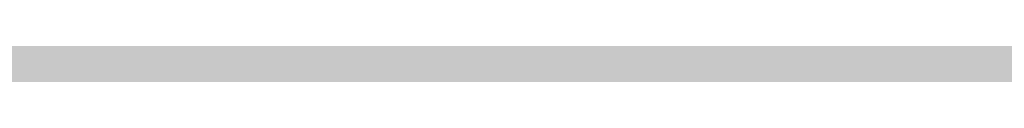
# Model space of a CAD drawing. Units: inches. Extents: x 2091 to 2899, y 967 to 2217.
# Tile 228 of 256: x 2203.4104 to 2203.7172, y 1152.2538 to 1152.2605. Entities that reach past the tile are written whole.
import ezdxf

# ---------------------------------------------------------------- set-up
doc = ezdxf.new("R2010")
doc.units = ezdxf.units.IN
doc.layers.add('A-WALL-PATT', color=141, linetype='Continuous', lineweight=13, true_color=0xadddf7)

msp = doc.modelspace()

# ---------------------------------------------------------------- hatches: boundary and pattern name
at = {"layer": 'A-WALL-PATT'}
h = msp.add_hatch(color=256, dxfattribs=at)
h.dxf.hatch_style = 1
h.paths.add_polyline_path([(2803.1436, 2050.91906), (2203.1436, 2050.91906), (2203.1436, 1090.91906), (2803.1436, 1090.91906)])
h.paths.add_polyline_path([(2635.79885, 1147.54046), (2674.52405, 1147.54046, 0.376086), (2678.52967, 1152.8802), (2678.52967, 1159.55647, 0.333335), (2674.52432, 1163.56185), (2674.52432, 1163.56185), (2674.52432, 1192.93439), (2635.80597, 1192.93439), (2597.08762, 1192.93439), (2597.08762, 1163.56185, 0.333335), (2593.08228, 1159.55647), (2593.08228, 1152.8802, 0.376086), (2597.08789, 1147.54046)], flags=0)
h.paths.add_polyline_path([(2436.01043, 1278.24078, 0.000483), (2435.95264, 1278.21503, -0.001328), (2435.93563, 1278.11169, -0.001711), (2436.11644, 1278.04076, 0.002185)], flags=0)
h.paths.add_polyline_path([(2794.1436, 1143.41906), (2794.1436, 1347.41906), (2543.37017, 1347.41906), (2543.37017, 1351.91906), (2794.1436, 1351.91906), (2794.1436, 1392.71355), (2793.9474, 1392.71355), (2793.9474, 1473.5369), (2794.1436, 1473.5369), (2794.1436, 1531.91906), (2650.1436, 1531.91906), (2650.1436, 1536.41906), (2794.1436, 1536.41906), (2794.1436, 1692.41906), (2609.37561, 1692.41906), (2609.37561, 1644.41906), (2604.87561, 1644.41906), (2604.87561, 1744.91906), (2609.37561, 1744.91906), (2609.37561, 1696.91906), (2794.1436, 1696.91906), (2794.1436, 1780.91906), (2609.6436, 1780.91906), (2493.87561, 1780.91906), (2493.87561, 1785.41906), (2609.6436, 1785.41906), (2794.1436, 1785.41906), (2794.1436, 1847.93882), (2793.95122, 1847.93882), (2793.95122, 1928.76217), (2794.1436, 1928.76217), (2794.1436, 1941.41906), (2614.1436, 1941.41906), (2614.1436, 1821.41906), (2609.6436, 1821.41906), (2609.6436, 1941.41906), (2392.1436, 1941.41906), (2392.1436, 1819.91906), (2387.6436, 1819.91906), (2387.6436, 1941.41906), (2212.1436, 1941.41906), (2212.1436, 1783.91906), (2392.1436, 1783.91906), (2392.1436, 1780.91906), (2212.1436, 1780.91906), (2212.1436, 1629.41906), (2387.6436, 1629.41906), (2387.6436, 1744.91906), (2392.1436, 1744.91906), (2392.1436, 1627.91906), (2317.1436, 1627.91906), (2317.1436, 1551.41906), (2317.1436, 1536.41906), (2459.38359, 1536.41906), (2459.38359, 1602.39648), (2463.88359, 1602.39648), (2463.88359, 1531.91906), (2456.6436, 1531.91906), (2456.6436, 1529.91906), (2452.1436, 1529.91906), (2452.1436, 1531.91906), (2312.6436, 1531.91906), (2312.6436, 1551.41906), (2306.1436, 1551.41906), (2306.1436, 1555.91906), (2308.1436, 1555.91906), (2308.1436, 1551.41906), (2312.6436, 1551.41906), (2312.6436, 1627.91906), (2212.1436, 1627.91906), (2212.1436, 1555.91906), (2270.1436, 1555.91906), (2270.1436, 1551.41906), (2212.1436, 1551.41906), (2212.1436, 1351.91906), (2272.1436, 1351.91906), (2272.1436, 1347.41906), (2212.1436, 1347.41906), (2212.1436, 1275.41906), (2308.1436, 1275.41906), (2308.1436, 1351.91906), (2452.1436, 1351.91906), (2452.1436, 1493.91906), (2456.6436, 1493.91906), (2456.6436, 1347.41906), (2312.6436, 1347.41906), (2312.6436, 1270.91906), (2212.1436, 1270.91906), (2212.1436, 1099.91906), (2281.23752, 1099.91906), (2282.87104, 1110.9138), (2282.00834, 1116.9966), (2278.55774, 1121.4204), (2268.20564, 1128.0562), (2272.08764, 1128.0562), (2273.81294, 1131.927), (2279.42034, 1134.6919), (2285.02784, 1135.2449), (2287.61584, 1137.4568), (2288.04714, 1138.0098), (2289.34114, 1140.7747), (2291.06654, 1139.6687), (2292.36054, 1135.2449), (2295.37984, 1136.9038), (2296.24254, 1135.7979), (2297.10524, 1133.033), (2300.12464, 1138.0098), (2303.14394, 1138.0098), (2304.43794, 1135.7979), (2303.14394, 1133.586), (2306.59464, 1134.6919), (2307.88874, 1133.033), (2310.90804, 1135.2449), (2313.92744, 1134.1389), (2315.62686, 1132.4271), (2308.32004, 1117.5496), (2290.20384, 1109.8079), (2288.90984, 1103.1721), (2289.27231, 1099.91906), (2434.91823, 1099.91906), (2431.59323, 1124.78806), (2429.93023, 1169.55306), (2430.92718, 1240.51969), (2435.65893, 1238.18613), (2437.13523, 1196.55406), (2438.79823, 1143.97306), (2442.67823, 1111.99806), (2446.55823, 1099.91906), (2794.1436, 1099.91906), (2794.1436, 1138.91906), (2548.03245, 1138.91906), (2548.03245, 1143.41906), (2548.03245, 1148.81906), (2546.66846, 1148.03156), (2528.68569, 1179.17862, 0.256256), (2512.03245, 1148.81906), (2512.03245, 1143.41906), (2512.03245, 1138.91906), (2507.53245, 1138.91906), (2507.53245, 1143.41906), (2507.53245, 1148.81906, 0.256256), (2490.8792, 1179.17862), (2472.89644, 1148.03156), (2471.53245, 1148.81906), (2471.53245, 1143.41906), (2467.03245, 1143.41906), (2467.03245, 1269.94579, 0.039061), (2460.90999, 1273.58006), (2467.03245, 1273.58006), (2467.03245, 1286.32536, 0.014511), (2465.21619, 1286.76191), (2467.03245, 1287.05258), (2467.03245, 1323.41906), (2471.53245, 1323.41906), (2471.53245, 1148.81906), (2489.53245, 1179.99597), (2490.89644, 1179.20847), (2490.8792, 1179.17862, -0.256256), (2507.53245, 1148.81906), (2507.53245, 1143.41906), (2512.03245, 1143.41906), (2512.03245, 1148.81906, -0.256256), (2528.68569, 1179.17862), (2528.66846, 1179.20847), (2530.03245, 1179.99597), (2548.03245, 1148.81906), (2548.03245, 1143.41906)], flags=16)
h.paths.add_polyline_path([(2607.76855, 1200.94508), (2607.76855, 1265.03063), (2597.08762, 1281.05201), (2619.78459, 1281.05201), (2627.79528, 1337.12686), (2635.79885, 1337.12686), (2643.81666, 1337.12686), (2651.82736, 1281.05201), (2674.52432, 1281.05201), (2663.8434, 1265.03063), (2663.8434, 1200.94508), (2635.80597, 1200.94508)], flags=0)
edge = h.paths.add_edge_path(flags=0)
edge.add_ellipse((13303.89622, 1272.99872), major_axis=(-10595.31304, 0), ratio=0.84230387009, start_angle=0.628237219, end_angle=0.6465541, ccw=False)
edge.add_ellipse((2711.70045, 1156.85268), major_axis=(2.21977, 0), ratio=0.8423039, start_angle=111.53524, end_angle=180.62824, ccw=False)
edge.add_ellipse((13303.15629, 1272.99872), major_axis=(-10593.02631, 0), ratio=0.84230386954, start_angle=0.528271472, end_angle=0.646554097, ccw=False)
edge.add_line((2710.7646, 1175.3333), (2710.12999, 1175.3333))
edge.add_ellipse((2710.12999, 1176.57978), major_axis=(1.47985, 0), ratio=0.8423039, start_angle=180, end_angle=270, ccw=False)
edge.add_line((2708.65014, 1176.57978), (2708.65014, 1200.78291))
edge.add_ellipse((2710.12999, 1200.78291), major_axis=(1.47985, 0), ratio=0.8423039, start_angle=90, end_angle=180, ccw=False)
edge.add_line((2710.12999, 1202.02939), (2710.46508, 1202.02939))
edge.add_ellipse((13303.15629, 1272.99872), major_axis=(-10593.02631, 0), ratio=0.84230386954, start_angle=-0.090229089, end_angle=0.383866779, ccw=False)
edge.add_ellipse((2710.12999, 1290.92703), major_axis=(-1.47985, 0), ratio=0.8423039, start_angle=0, end_angle=90, ccw=False)
edge.add_line((2708.65014, 1290.92703), (2708.65014, 1315.13017))
edge.add_ellipse((2710.12999, 1315.13017), major_axis=(-1.47985, 0), ratio=0.8423039, start_angle=-90, end_angle=0, ccw=False)
edge.add_line((2710.12999, 1316.37665), (2710.70631, 1316.37665))
edge.add_ellipse((3238.40172, 1296.28957), major_axis=(528.234, 0), ratio=0.84230387, start_angle=176.3495724, end_angle=177.8200497, ccw=False)
edge.add_ellipse((2775.06304, 1071.4507), major_axis=(313.30776, 0), ratio=0.84230387, start_angle=102.1259656, end_angle=103.780529, ccw=False)
edge.add_ellipse((2775.06304, 1078.3057), major_axis=(-305.30289, 0), ratio=0.84230387, start_angle=-79.790461, end_angle=-77.5553727, ccw=False)
edge.add_ellipse((2695.14177, 1541.97538), major_axis=(-250.96022, 0), ratio=0.84230387, start_angle=99.256566, end_angle=102.5549326)
edge.add_line((2741.41033, 1334.21426), (2747.13255, 1337.37848))
edge.add_ellipse((2747.53862, 1336.85748), major_axis=(-0.73992, 0), ratio=0.842304, start_angle=270, end_angle=307.93313, ccw=False)
edge.add_ellipse((2747.53862, 1336.85748), major_axis=(-0.73992, 0), ratio=0.842304, start_angle=232.06687, end_angle=270, ccw=False)
edge.add_line((2747.94469, 1337.37848), (2753.66691, 1334.21426))
edge.add_ellipse((2799.93547, 1541.97538), major_axis=(250.96022, 0), ratio=0.84230387, start_angle=257.4450674, end_angle=260.743434)
edge.add_ellipse((2720.01419, 1078.3057), major_axis=(305.30289, 0), ratio=0.84230387, start_angle=77.5553727, end_angle=79.790461, ccw=False)
edge.add_ellipse((2720.01419, 1071.4507), major_axis=(-313.30776, 0), ratio=0.84230387, start_angle=256.219471, end_angle=257.8740344, ccw=False)
edge.add_ellipse((2256.67551, 1296.28957), major_axis=(-528.234, 0), ratio=0.84230387, start_angle=182.1799503, end_angle=183.6504276, ccw=False)
edge.add_line((2784.37092, 1316.37665), (2784.94725, 1316.37665))
edge.add_ellipse((2784.94725, 1315.13017), major_axis=(1.47985, 0), ratio=0.8423039, start_angle=0, end_angle=90, ccw=False)
edge.add_line((2786.42709, 1315.13017), (2786.42709, 1290.92703))
edge.add_ellipse((2784.94725, 1290.92703), major_axis=(1.47985, 0), ratio=0.8423039, start_angle=270, end_angle=360, ccw=False)
edge.add_ellipse((-7808.07906, 1272.99872), major_axis=(10593.02631, 0), ratio=0.84230386954, start_angle=-0.383866779, end_angle=0.090229089, ccw=False)
edge.add_line((2784.61216, 1202.02939), (2784.94725, 1202.02939))
edge.add_ellipse((2784.94725, 1200.78291), major_axis=(1.47985, 0), ratio=0.8423039, start_angle=0, end_angle=90, ccw=False)
edge.add_line((2786.42709, 1200.78291), (2786.42709, 1176.57978))
edge.add_ellipse((2784.94725, 1176.57978), major_axis=(-1.47985, 0), ratio=0.8423039, start_angle=90, end_angle=180, ccw=False)
edge.add_line((2784.94725, 1175.3333), (2784.31264, 1175.3333))
edge.add_ellipse((-7808.07906, 1272.99872), major_axis=(10593.02631, 0), ratio=0.84230386954, start_angle=-0.618643196, end_angle=-0.528271472, ccw=False)
edge.add_ellipse((2783.37678, 1156.85268), major_axis=(-2.21977, 0), ratio=0.8423039, start_angle=179.37176, end_angle=248.46476, ccw=False)
edge.add_ellipse((-7808.81898, 1272.99872), major_axis=(-10595.31304, 0), ratio=0.84230386576, start_angle=179.353445923, end_angle=179.371762803, ccw=False)
edge.add_ellipse((2780.2973, 1153.50079), major_axis=(-5.24643, 0), ratio=0.8423039, start_angle=90, end_angle=179.35345, ccw=False)
edge.add_line((2780.2973, 1149.08171), (2714.77993, 1149.08171))
edge.add_ellipse((2714.77993, 1153.50079), major_axis=(5.24643, 0), ratio=0.8423039, start_angle=180.64655, end_angle=270, ccw=False)
edge = h.paths.add_edge_path(flags=0)
edge.add_line((2718.18737, 1151.00783), (2718.18737, 1170.47236))
edge.add_ellipse((2721.14706, 1170.47236), major_axis=(-2.95969, 0), ratio=0.8423039, start_angle=-90, end_angle=0, ccw=False)
edge.add_line((2721.14706, 1172.96532), (2773.93017, 1172.96532))
edge.add_ellipse((2773.93017, 1170.47236), major_axis=(-2.95969, 0), ratio=0.8423039, start_angle=180, end_angle=270, ccw=False)
edge.add_line((2776.88987, 1170.47236), (2776.88987, 1151.00783))
edge.add_line((2776.88987, 1151.00783), (2718.18737, 1151.00783))
edge = h.paths.add_edge_path(flags=0)
edge.add_line((2718.18737, 1180.23415), (2718.18737, 1199.05783))
edge.add_ellipse((2747.53862, 1320.39864), major_axis=(147.01792, 0), ratio=0.84230387, start_angle=256.4018653, end_angle=283.5981347)
edge.add_line((2776.88987, 1199.05783), (2776.88987, 1180.23415))
edge.add_ellipse((2747.53862, 1301.57496), major_axis=(147.01792, 0), ratio=0.84230387, start_angle=256.4018653, end_angle=283.5981347, ccw=False)
edge = h.paths.add_edge_path(flags=0)
edge.add_ellipse((13303.15629, 1272.99872), major_axis=(-10591.54646, 0), ratio=0.84230386955, start_angle=0.055594314, end_angle=0.377764194, ccw=False)
edge.add_line((2711.61686, 1262.72171), (2715.66741, 1249.4954))
edge.add_ellipse((6413.89196, 1241.69192), major_axis=(-3698.23616, 0), ratio=0.8423038695, start_angle=-0.12089737, end_angle=0.36407635)
edge.add_line((2715.76104, 1218.19245), (2711.93431, 1203.16736))
edge = h.paths.add_edge_path(flags=0)
edge.add_line((2718.18737, 1251.07457), (2716.00249, 1267.45044))
edge.add_ellipse((2742.15117, 1202.18954), major_axis=(81.77258, 0), ratio=0.84230387, start_angle=94.277421, end_angle=111.8349538, ccw=False)
edge.add_line((2737.00975, 1270.93063), (2758.06748, 1270.93063))
edge.add_ellipse((2752.92606, 1202.18954), major_axis=(81.77258, 0), ratio=0.84230387, start_angle=68.1650462, end_angle=85.722579, ccw=False)
edge.add_line((2779.07475, 1267.45044), (2776.88987, 1251.07457))
edge.add_ellipse((2750.33806, 1187.88536), major_axis=(79.57966, 0), ratio=0.84230387, start_angle=67.2080851, end_angle=85.1299304)
edge.add_line((2756.03466, 1254.74366), (2739.04258, 1254.74366))
edge.add_ellipse((2744.73917, 1187.88536), major_axis=(79.57966, 0), ratio=0.84230387, start_angle=94.8700696, end_angle=112.7919149)
edge = h.paths.add_edge_path(flags=0)
edge.add_line((2783.14293, 1203.16736), (2779.31619, 1218.19245))
edge.add_ellipse((-918.81473, 1241.69192), major_axis=(3698.23616, 0), ratio=0.8423038695, start_angle=-0.36407635, end_angle=0.12089737)
edge.add_line((2779.40983, 1249.4954), (2783.46037, 1262.72171))
edge.add_ellipse((-7808.07906, 1272.99872), major_axis=(-10591.54646, 0), ratio=0.84230386954, start_angle=179.622235806, end_angle=179.944405687, ccw=False)
edge = h.paths.add_edge_path(flags=0)
edge.add_ellipse((2734.20089, 1286.69044), major_axis=(-0.35661, 6.34008), ratio=0.6038336, start_angle=89.002014, end_angle=253.657408, ccw=False)
edge.add_line((2730.369, 1286.54181), (2730.369, 1301.35198))
edge.add_line((2730.369, 1301.35198), (2735.91331, 1305.2148))
edge.add_ellipse((2736.38492, 1304.73456), major_axis=(0.73992, 0), ratio=0.842304, start_angle=90, end_angle=134.48021, ccw=False)
edge.add_line((2736.38492, 1305.3578), (2738.03278, 1305.3578))
edge.add_line((2738.03278, 1305.3578), (2738.03278, 1307.70793))
edge.add_ellipse((2794.20164, 1307.70793), major_axis=(56.16886, 0), ratio=0.84230387, start_angle=150.56143, end_angle=180, ccw=False)
edge.add_ellipse((2700.87559, 1307.70793), major_axis=(-56.16886, 0), ratio=0.84230387, start_angle=180, end_angle=209.43857, ccw=False)
edge.add_line((2757.04445, 1307.70793), (2757.04445, 1305.3578))
edge.add_line((2757.04445, 1305.3578), (2758.69232, 1305.3578))
edge.add_ellipse((2758.69232, 1304.73456), major_axis=(-0.73992, 0), ratio=0.842304, start_angle=225.51979, end_angle=270, ccw=False)
edge.add_line((2759.16392, 1305.2148), (2764.70823, 1301.35198))
edge.add_line((2764.70823, 1301.35198), (2764.70823, 1286.54181))
edge.add_ellipse((2760.87634, 1286.69044), major_axis=(0.35661, 6.34008), ratio=0.6038336, start_angle=106.342592, end_angle=270.997986, ccw=False)
edge.add_line((2757.04445, 1285.79709), (2757.04445, 1307.70793))
edge.add_ellipse((2700.87559, 1307.70793), major_axis=(-56.16886, 0), ratio=0.84230387, start_angle=180, end_angle=209.43857)
edge.add_ellipse((2794.20164, 1307.70793), major_axis=(56.16886, 0), ratio=0.84230387, start_angle=150.56143, end_angle=180)
edge.add_line((2738.03278, 1307.70793), (2738.03278, 1285.79709))
h.paths.add_polyline_path([(2417.81227, 1104.4497), (2413.49227, 1102.5297), (2410.61227, 1103.9697), (2409.17227, 1106.3697), (2407.25227, 1107.3297), (2406.29227, 1109.7297), (2405.33227, 1114.0497), (2405.33227, 1117.8897), (2406.29227, 1120.1297), (2407.25227, 1119.8097), (2408.84832, 1118.32766), (2410.17395, 1119.42417), (2410.21127, 1120.4057), (2411.04073, 1121.41905), (2410.69927, 1119.8587), (2410.17395, 1119.42417), (2410.08845, 1117.17611), (2411.13284, 1116.20632), (2413.97227, 1119.3297), (2416.85227, 1120.7697), (2416.86972, 1120.79878), (2417.03507, 1119.40512), (2417.89621, 1118.14338), (2418.29227, 1118.3697), (2419.54445, 1120.03927), (2419.36092, 1118.38749), (2419.03211, 1119.35615), (2418.39894, 1118.51193), (2419.25227, 1114.5297), (2418.79409, 1107.19879)], flags=0)
h.paths.add_polyline_path([(2508.87017, 1347.41906), (2508.37017, 1347.41906), (2508.37017, 1351.91906), (2508.87017, 1351.91906)], flags=0)
h.paths.add_polyline_path([(2473.37017, 1347.41906), (2472.37017, 1347.41906), (2467.87017, 1347.41906), (2467.87017, 1455.41906), (2472.37017, 1455.41906), (2472.37017, 1352.41906), (2473.37017, 1352.41906)], flags=0)
h.paths.add_polyline_path([(2352.10624, 1217.4462), (2349.22624, 1218.8862), (2347.78624, 1221.2862), (2345.86624, 1222.2462), (2344.90624, 1224.6462), (2343.94624, 1228.9662), (2343.94624, 1232.8062), (2344.90624, 1235.0462), (2345.86624, 1234.7262), (2347.46229, 1233.24415), (2348.78792, 1234.34066), (2348.82524, 1235.3222), (2349.6547, 1236.33555), (2349.31324, 1234.7752), (2348.78792, 1234.34066), (2348.70242, 1232.0926), (2349.74681, 1231.12282), (2352.58624, 1234.2462), (2355.46624, 1235.6862), (2355.48369, 1235.71528), (2355.64904, 1234.32161), (2356.51018, 1233.05988), (2356.90624, 1233.2862), (2358.15842, 1234.95576), (2357.97489, 1233.30398), (2357.64608, 1234.27264), (2357.01291, 1233.42842), (2357.86624, 1229.4462), (2357.40806, 1222.11529), (2356.42624, 1219.3662)], flags=0)
h.paths.add_polyline_path([(2348.2968, 1112.22442), (2347.0138, 1112.31042), (2345.5298, 1114.12742), (2345.7318, 1115.85842), (2346.8118, 1116.98242), (2346.8118, 1114.64642), (2345.8668, 1114.21442), (2346.8798, 1114.30042)], flags=0)
h.paths.add_polyline_path([(2347.0138, 1110.92642), (2346.2718, 1110.49342), (2346.6098, 1111.18642)], flags=0)
h.paths.add_polyline_path([(2345.8668, 1118.19442), (2345.5298, 1117.32942), (2343.7078, 1118.02142), (2344.3828, 1118.62642)], flags=0)
h.paths.add_polyline_path([(2346.6768, 1109.28242), (2346.0698, 1108.07142), (2345.8668, 1110.06142)], flags=0)
h.paths.add_polyline_path([(2345.0568, 1119.75142), (2343.6398, 1119.75142), (2343.9778, 1121.13542)], flags=0)
h.paths.add_polyline_path([(2345.2598, 1116.55042), (2345.1248, 1115.85842), (2344.9218, 1115.68542), (2344.7198, 1116.37742)], flags=0)
h.paths.add_polyline_path([(2345.6648, 1112.31042), (2345.4618, 1111.53242), (2344.0448, 1111.96442), (2344.6518, 1112.57042)], flags=0)
h.paths.add_polyline_path([(2345.1918, 1113.34942), (2344.4498, 1113.86842), (2344.7198, 1114.38742)], flags=0)
h.paths.add_polyline_path([(2344.6518, 1116.80942), (2344.1798, 1115.68542), (2344.6518, 1115.33942), (2343.9098, 1114.90642), (2343.0328, 1115.94442), (2343.6398, 1116.46342)], flags=0)
h.paths.add_polyline_path([(2345.8668, 1106.68642), (2344.9898, 1105.56242), (2344.5168, 1106.60042)], flags=0)
h.paths.add_polyline_path([(2344.8548, 1110.06142), (2344.5168, 1109.28242), (2344.1128, 1109.71542)], flags=0)
h.paths.add_polyline_path([(2344.0448, 1113.52242), (2343.4378, 1113.08942), (2342.7628, 1113.95442)], flags=0)
h.paths.add_polyline_path([(2344.3148, 1111.01242), (2342.9648, 1110.32042), (2342.9648, 1111.09942)], flags=0)
h.paths.add_polyline_path([(2345.1248, 1104.69742), (2344.5848, 1103.74542), (2344.4498, 1104.26442)], flags=0)
h.paths.add_polyline_path([(2342.8298, 1121.22242), (2341.7498, 1120.53042), (2340.5358, 1121.04942), (2340.1308, 1121.82842), (2340.6708, 1122.95242), (2341.1428, 1121.82842), (2341.6148, 1122.00142)], flags=0)
h.paths.add_polyline_path([(2342.9648, 1119.75142), (2343.0328, 1118.45342), (2342.0878, 1118.02142), (2342.0198, 1119.49142)], flags=0)
h.paths.add_polyline_path([(2342.6948, 1116.89642), (2341.9528, 1116.63642), (2342.0198, 1117.32942)], flags=0)
h.paths.add_polyline_path([(2343.0328, 1112.22442), (2342.0198, 1111.79142), (2341.5478, 1112.22442), (2342.3578, 1113.34942)], flags=0)
h.paths.add_polyline_path([(2343.7748, 1104.43742), (2342.6278, 1102.88042), (2342.6948, 1104.61042), (2343.4378, 1105.12942)], flags=0)
h.paths.add_polyline_path([(2342.0198, 1115.07942), (2340.8058, 1115.51242), (2340.9408, 1116.37742)], flags=0)
h.paths.add_polyline_path([(2341.4808, 1120.09742), (2341.4808, 1119.40542), (2341.0758, 1119.57842), (2341.1428, 1120.09742)], flags=0)
h.paths.add_polyline_path([(2341.8178, 1114.47342), (2340.9408, 1113.08942), (2340.8058, 1114.56042)], flags=0)
h.paths.add_polyline_path([(2341.1428, 1118.54042), (2340.9408, 1116.98242), (2339.0508, 1117.67542), (2339.0508, 1118.62642)], flags=0)
h.paths.add_polyline_path([(2342.6948, 1101.66842), (2341.9528, 1101.84142), (2342.5598, 1102.36142)], flags=0)
h.paths.add_polyline_path([(2340.3328, 1119.66542), (2338.4438, 1119.57842), (2337.9038, 1120.35742), (2339.6578, 1120.61642)], flags=0)
h.paths.add_polyline_path([(2340.3328, 1115.33942), (2340.0628, 1113.69542), (2339.3878, 1115.33942)], flags=0)
h.paths.add_polyline_path([(2341.8178, 1103.83142), (2341.5478, 1102.88042), (2341.1428, 1103.65842)], flags=0)
h.paths.add_polyline_path([(2339.0508, 1122.86642), (2337.2958, 1121.82842), (2337.0938, 1123.12542), (2337.7688, 1123.81842)], flags=0)
h.paths.add_polyline_path([(2339.1178, 1121.74142), (2338.8478, 1121.22242), (2338.1738, 1121.04942), (2338.3758, 1121.56842)], flags=0)
h.paths.add_polyline_path([(2339.1858, 1119.31942), (2338.6458, 1118.71342), (2338.2408, 1118.10742), (2338.2408, 1118.88642)], flags=0)
h.paths.add_polyline_path([(2341.1428, 1101.92842), (2340.6028, 1101.23642), (2340.0628, 1101.84142), (2340.6028, 1102.36142)], flags=0)
h.paths.add_polyline_path([(2337.6338, 1117.76142), (2336.6208, 1118.28042), (2337.2958, 1118.97242)], flags=0)
h.paths.add_polyline_path([(2336.8238, 1119.57842), (2334.7988, 1118.97242), (2335.2038, 1120.35742), (2336.5538, 1120.87642)], flags=0)
h.paths.add_polyline_path([(2339.1178, 1100.45742), (2337.3638, 1100.54342), (2336.7558, 1101.23642)], flags=0)
h.paths.add_polyline_path([(2336.3508, 1122.43342), (2336.0138, 1121.91442), (2334.9338, 1122.43342), (2334.5288, 1123.47142), (2335.7438, 1122.77942)], flags=0)
h.paths.add_polyline_path([(2334.7318, 1120.87642), (2334.2588, 1120.35742), (2334.0568, 1120.78942), (2334.5968, 1121.30842)], flags=0)
h.paths.add_polyline_path([(2334.4618, 1122.17442), (2332.5718, 1121.30842), (2331.3568, 1122.17442), (2332.0998, 1122.86642)], flags=0)
h.paths.add_polyline_path([(2334.2588, 1118.54042), (2333.3818, 1118.45342), (2333.6518, 1119.31942)], flags=0)
h.paths.add_polyline_path([(2335.5418, 1102.27442), (2334.1918, 1102.62042), (2335.2718, 1103.31242)], flags=0)
h.paths.add_polyline_path([(2332.7068, 1119.66542), (2331.6948, 1120.44342), (2332.5048, 1120.78942)], flags=0)
h.paths.add_polyline_path([(2334.7318, 1101.14942), (2333.5168, 1101.58242), (2333.9888, 1101.75542)], flags=0)
h.paths.add_polyline_path([(2332.6398, 1116.63642), (2331.0868, 1116.29042), (2331.9648, 1118.19442)], flags=0)
h.paths.add_polyline_path([(2330.7498, 1121.56842), (2330.2768, 1120.27042), (2328.5228, 1119.31942), (2328.9948, 1121.04942)], flags=0)
h.paths.add_polyline_path([(2330.7498, 1118.62642), (2330.0078, 1117.50242), (2329.8728, 1118.02142)], flags=0)
h.paths.add_polyline_path([(2332.0998, 1102.36142), (2330.5468, 1102.01442), (2331.6948, 1102.96642)], flags=0)
h.paths.add_polyline_path([(2329.5348, 1113.60842), (2329.0628, 1112.31042), (2328.5898, 1113.34942)], flags=0)
h.paths.add_polyline_path([(2328.3878, 1117.84842), (2327.5098, 1116.55042), (2327.1728, 1117.76142)], flags=0)
h.paths.add_polyline_path([(2329.7378, 1106.51342), (2329.5348, 1105.30242), (2328.2528, 1106.08142)], flags=0)
h.paths.add_polyline_path([(2328.6578, 1114.38742), (2328.0498, 1114.12742), (2328.3198, 1114.90642)], flags=0)
h.paths.add_polyline_path([(2328.3198, 1112.22442), (2327.1058, 1112.13742), (2326.7008, 1112.65642)], flags=0)
h.paths.add_polyline_path([(2326.9028, 1115.25242), (2326.7008, 1114.12742), (2325.2158, 1113.60842), (2326.0928, 1115.33942)], flags=0)
h.paths.add_polyline_path([(2326.6328, 1108.33042), (2326.0928, 1107.37942), (2325.8908, 1108.50342), (2326.4978, 1109.10942)], flags=0)
h.paths.add_polyline_path([(2615.1436, 1531.91906), (2609.6436, 1531.91906), (2609.6436, 1620.41906), (2614.1436, 1620.41906), (2614.1436, 1536.41906), (2615.1436, 1536.41906)], flags=0)
h.paths.add_polyline_path([(2545.1436, 1563.41906), (2464.1436, 1563.41906), (2464.1436, 1632.41906), (2509.1436, 1632.41906), (2509.1436, 1627.91906), (2509.1436, 1603.91906), (2468.6436, 1603.91906), (2468.6436, 1567.91906), (2540.6436, 1567.91906), (2540.6436, 1591.91906), (2545.1436, 1591.91906)], flags=0)
h.paths.add_polyline_path([(2388.96905, 1549.98573), (2357.43418, 1549.98573), (2357.43418, 1623.36078), (2399.36278, 1623.36078), (2435.68947, 1623.36078), (2435.59255, 1602.55927), (2435.59255, 1602.39648), (2388.96905, 1602.39648)], flags=0)
h.paths.add_polyline_path([(2388.88063, 1555.80915), (2374.90443, 1555.80915), (2374.90443, 1600.57156), (2374.90443, 1615.45765), (2406.35088, 1615.45765), (2406.35088, 1618.93943), (2412.17429, 1615.45765), (2406.35088, 1611.97586), (2406.35088, 1615.45765), (2388.88063, 1615.45765)], flags=0)
h.paths.add_polyline_path([(2568.87561, 1644.41906), (2453.37561, 1644.41906), (2453.37561, 1785.41906), (2457.87561, 1785.41906), (2457.87561, 1648.91906), (2568.87561, 1648.91906)], flags=0)
h.paths.add_polyline_path([(2212.1436, 1945.91906), (2212.1436, 2041.91906), (2794.1436, 2041.91906), (2794.1436, 1945.91906)], flags=16)
h.paths.add_polyline_path([(2271.08273, 1964.31724), (2776.85297, 1964.31724), (2776.85297, 2037.16962), (2271.08273, 2037.16962)], flags=8)
h.paths.add_polyline_path([(2380.64929, 1536.82414), (2461.04081, 1536.82414), (2461.04081, 1554.65259), (2380.64929, 1554.65259)], flags=8)
h.paths.add_polyline_path([(2240.75571, 1609.72545), (2309.18583, 1609.72545), (2309.18583, 1617.6982), (2240.75571, 1617.6982)], flags=8)
h.paths.add_polyline_path([(2212.67726, 1313.5041), (2282.59152, 1313.5041), (2282.59152, 1322.74524), (2212.67726, 1322.74524)], flags=8)
h.paths.add_polyline_path([(2457.11198, 1114.77857), (2558.48158, 1114.77857), (2558.48158, 1142.21968), (2457.11198, 1142.21968)], flags=8)
h.paths.add_polyline_path([(2473.44234, 1273.01007), (2604.64123, 1273.01007), (2604.64123, 1318.34693), (2473.44234, 1318.34693)], flags=8)
h.paths.add_polyline_path([(2638.8763, 1626.97743), (2684.25037, 1627.97674), (2684.03848, 1637.59749), (2638.66442, 1636.59819)], flags=8)
h.paths.add_polyline_path([(2537.59055, 1453.79345), (2628.38955, 1453.79345), (2628.38955, 1475.34481), (2537.59055, 1475.34481)], flags=8)
h.paths.add_polyline_path([(2504.13764, 1714.6324), (2554.64719, 1714.6324), (2554.64719, 1730.23771), (2504.13764, 1730.23771)], flags=8)
h.paths.add_polyline_path([(2487.50118, 1575.65187), (2535.09712, 1575.65187), (2535.09712, 1598.37765), (2487.50118, 1598.37765)], flags=8)
h.paths.add_polyline_path([(2709.0994, 1735.71028), (2740.0166, 1735.71028), (2740.0166, 1749.93764), (2709.0994, 1749.93764)], flags=8)
h.paths.add_polyline_path([(2442.43842, 1792.17166), (2564.72884, 1792.17166), (2564.72884, 1842.00016), (2442.43842, 1842.00016)], flags=8)
h.paths.add_polyline_path([(2655.8158, 1809.64408), (2789.52014, 1806.6938), (2790.08498, 1832.29164), (2656.38064, 1835.24192)], flags=8)
h.paths.add_polyline_path([(2234.8427, 1797.72014), (2368.59285, 1794.76885), (2369.16072, 1820.50413), (2235.41056, 1823.45542)], flags=8)
h.paths.add_polyline_path([(2245.13847, 1644.00633), (2398.42773, 1640.6239), (2398.99484, 1666.32482), (2245.70557, 1669.70725)], flags=8)
h.paths.add_polyline_path([(2306.14285, 1431.16852), (2413.76831, 1428.79369), (2414.33315, 1454.39153), (2306.70768, 1456.76636)], flags=8)
h.paths.add_polyline_path([(2306.83458, 1458.23314), (2393.38048, 1456.32345), (2393.93281, 1481.35436), (2307.38691, 1483.26405)], flags=8)

doc.saveas('drawing.dxf')
